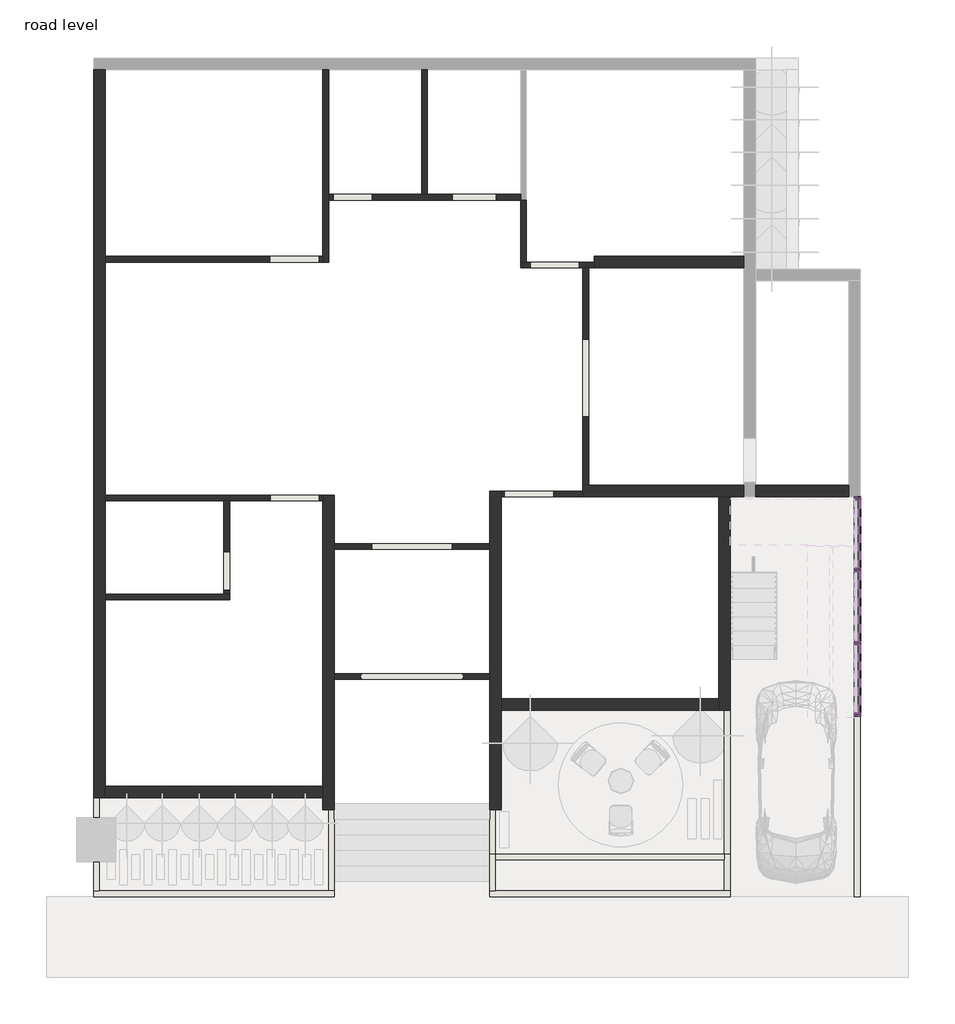
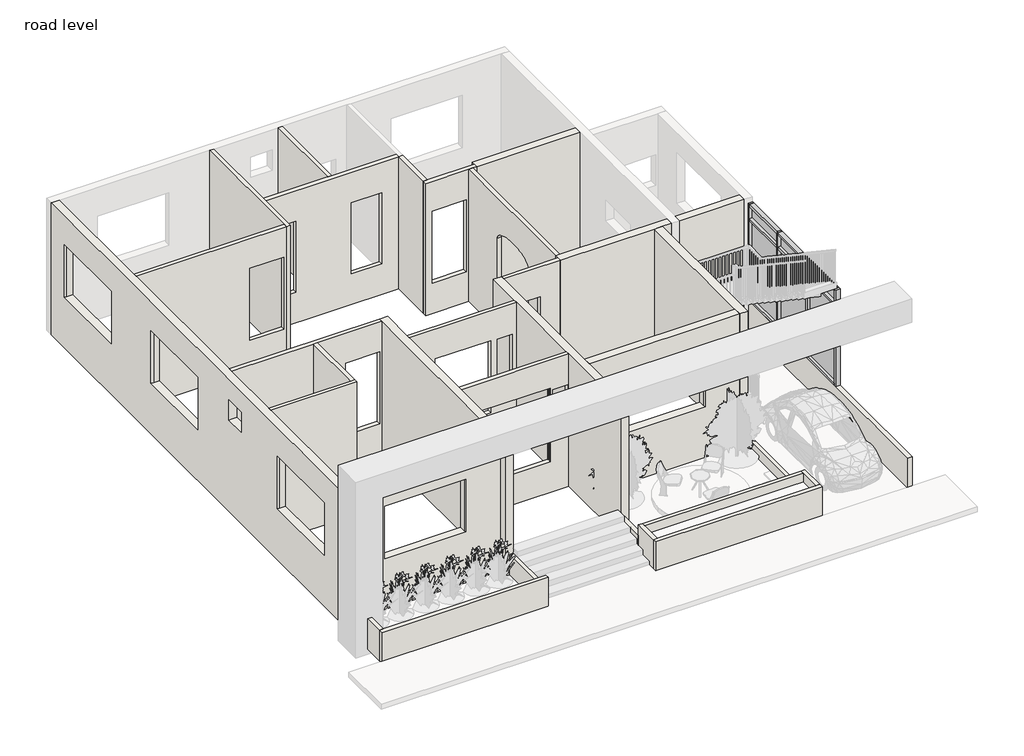
# One storey, part 1 of 3: 32 walls, 17 members, 6 plates.
"""IFC4 building model written with IfcOpenShell, lengths in millimetres."""

from ifc_helpers import new_model, si_unit, point, frame, origin, origin_with_axes, place, context, project, spatial, polyline, ellipse_curve, trimmed, outline, extrude, faceted_brep, transform, mapped, element, save
from ifc_brep_helpers import plane_surface, extruded_surface, advanced_brep
from components import member_97a07400, member_91c435ce, member_f0fea5a5, member_ffd4c858, member_64ac20db, member_08a74848, member_ee409385, member_15823cb3, system_panel_glazed_bd4b6abd, system_panel_glazed_9f7cb957, system_panel_glazed_bee7dd50, system_panel_glazed_ee0060d4

model = new_model("IFC4")

# Units and contexts
model_context = context("Model", 3, world=origin())
ifc_project = project(units=[si_unit("LENGTHUNIT", "METRE", prefix="MILLI")], contexts=[model_context])

# Site, building, storey
site = spatial("IfcSite", under=ifc_project)
building = spatial("IfcBuilding", under=site)
storey = spatial("IfcBuildingStorey", under=building, Name="road level", Elevation=0.0)

# Members
placement = place(None, origin())
member_shape = member_97a07400(model_context)
element("IfcMember", 1, ObjectType="Rectangular Mullion : 2.5\" x 5\" rectangular", at=placement, inside=storey, context=model_context, shape_type="MappedRepresentation", body=[
    mapped(member_shape, transform((-5177.1494093, 2444.9237487, 3810.0), x_axis=(0.0, 0.0, 1.0), y_axis=(-1.0, 0.0, 0.0), z_axis=(0.0, -1.0, 0.0))),
])
element("IfcMember", 2, ObjectType="Rectangular Mullion : 2.5\" x 5\" rectangular", at=placement, inside=storey, context=model_context, shape_type="MappedRepresentation", body=[
    mapped(member_shape, transform((-5177.1494093, 5283.3737486, 3810.0), x_axis=(0.0, 0.0, 1.0), y_axis=(-1.0, 0.0, 0.0), z_axis=(0.0, -1.0, 0.0))),
])
member_2_shape = member_91c435ce(model_context)
element("IfcMember", 3, ObjectType="Rectangular Mullion : 2.5\" x 5\" rectangular", at=placement, inside=storey, context=model_context, shape_type="MappedRepresentation", body=[
    mapped(member_2_shape, transform((-5177.1494093, 3848.2737488, 3810.0), x_axis=(0.0, 0.0, 1.0), y_axis=(-1.0, 0.0, 0.0), z_axis=(0.0, -1.0, 0.0))),
])
element("IfcMember", 4, ObjectType="Rectangular Mullion : 2.5\" x 5\" rectangular", at=placement, inside=storey, context=model_context, shape_type="MappedRepresentation", body=[
    mapped(member_shape, transform((-5177.1494093, 6623.2237487, 914.4), x_axis=(0.0, 0.0, -1.0), y_axis=(-1.0, 0.0, 0.0), z_axis=(0.0, 1.0, 0.0))),
])
element("IfcMember", 5, ObjectType="Rectangular Mullion : 2.5\" x 5\" rectangular", at=placement, inside=storey, context=model_context, shape_type="MappedRepresentation", body=[
    mapped(member_shape, transform((-5177.1494093, 3784.7737488, 914.4), x_axis=(0.0, 0.0, -1.0), y_axis=(-1.0, 0.0, 0.0), z_axis=(0.0, 1.0, 0.0))),
])
element("IfcMember", 6, ObjectType="Rectangular Mullion : 2.5\" x 5\" rectangular", at=placement, inside=storey, context=model_context, shape_type="MappedRepresentation", body=[
    mapped(member_2_shape, transform((-5177.1494093, 5219.8737486, 914.4), x_axis=(0.0, 0.0, -1.0), y_axis=(-1.0, 0.0, 0.0), z_axis=(0.0, 1.0, 0.0))),
])
member_3_shape = member_f0fea5a5(model_context)
element("IfcMember", 7, ObjectType="Rectangular Mullion : 2.5\" x 5\" rectangular", at=placement, inside=storey, context=model_context, shape_type="MappedRepresentation", body=[
    mapped(member_3_shape, transform((-5177.1494093, 5251.6237486, 914.4), x_axis=(0.0, -1.0, 0.0), y_axis=(-1.0, 0.0, 0.0), z_axis=(0.0, 0.0, -1.0))),
])
element("IfcMember", 8, ObjectType="Rectangular Mullion : 2.5\" x 5\" rectangular", at=placement, inside=storey, context=model_context, shape_type="MappedRepresentation", body=[
    mapped(member_3_shape, transform((-5177.1494093, 3816.5237488, 914.4), x_axis=(0.0, -1.0, 0.0), y_axis=(-1.0, 0.0, 0.0), z_axis=(0.0, 0.0, -1.0))),
])
member_4_shape = member_ffd4c858(model_context)
element("IfcMember", 9, ObjectType="Rectangular Mullion : 2.5\" x 5\" rectangular", at=placement, inside=storey, context=model_context, shape_type="MappedRepresentation", body=[
    mapped(member_4_shape, transform((-5177.1494093, 5251.6237486, 3352.8), x_axis=(0.0, -1.0, 0.0), y_axis=(-1.0, 0.0, 0.0), z_axis=(0.0, 0.0, -1.0))),
])
element("IfcMember", 10, ObjectType="Rectangular Mullion : 2.5\" x 5\" rectangular", at=placement, inside=storey, context=model_context, shape_type="MappedRepresentation", body=[
    mapped(member_4_shape, transform((-5177.1494093, 3816.5237488, 3352.8), x_axis=(0.0, -1.0, 0.0), y_axis=(-1.0, 0.0, 0.0), z_axis=(0.0, 0.0, -1.0))),
])
member_5_shape = member_64ac20db(model_context)
element("IfcMember", 11, ObjectType="Rectangular Mullion : 2.5\" x 5\" rectangular", at=placement, inside=storey, context=model_context, shape_type="MappedRepresentation", body=[
    mapped(member_5_shape, transform((-5177.1494093, 5283.3737486, 3352.8), x_axis=(0.0, 0.0, 1.0), y_axis=(-1.0, 0.0, 0.0), z_axis=(0.0, -1.0, 0.0))),
])
element("IfcMember", 12, ObjectType="Rectangular Mullion : 2.5\" x 5\" rectangular", at=placement, inside=storey, context=model_context, shape_type="MappedRepresentation", body=[
    mapped(member_5_shape, transform((-5177.1494093, 2444.9237487, 3352.8), x_axis=(0.0, 0.0, 1.0), y_axis=(-1.0, 0.0, 0.0), z_axis=(0.0, -1.0, 0.0))),
])
member_6_shape = member_08a74848(model_context)
element("IfcMember", 13, ObjectType="Rectangular Mullion : 2.5\" x 5\" rectangular", at=placement, inside=storey, context=model_context, shape_type="MappedRepresentation", body=[
    mapped(member_6_shape, transform((-5177.1494093, 3848.2737488, 3352.8), x_axis=(0.0, 0.0, 1.0), y_axis=(-1.0, 0.0, 0.0), z_axis=(0.0, -1.0, 0.0))),
])
member_7_shape = member_ee409385(model_context)
element("IfcMember", 14, ObjectType="Rectangular Mullion : 2.5\" x 5\" rectangular", at=placement, inside=storey, context=model_context, shape_type="MappedRepresentation", body=[
    mapped(member_7_shape, transform((-5177.1494093, 2381.4237487, 914.4), x_axis=(0.0, -1.0, 0.0), y_axis=(-1.0, 0.0, 0.0), z_axis=(0.0, 0.0, -1.0))),
])
member_8_shape = member_15823cb3(model_context)
element("IfcMember", 15, ObjectType="Rectangular Mullion : 2.5\" x 5\" rectangular", at=placement, inside=storey, context=model_context, shape_type="MappedRepresentation", body=[
    mapped(member_8_shape, transform((-5177.1494093, 6686.7237487, 3810.0), x_axis=(0.0, 1.0, 0.0), y_axis=(-1.0, 0.0, 0.0), z_axis=(0.0, 0.0, 1.0))),
])
element("IfcMember", 16, ObjectType="Rectangular Mullion : 2.5\" x 5\" rectangular", at=placement, inside=storey, context=model_context, shape_type="MappedRepresentation", body=[
    mapped(member_8_shape, transform((-5177.1494093, 2381.4237487, 3352.8), x_axis=(0.0, -1.0, 0.0), y_axis=(-1.0, 0.0, 0.0), z_axis=(0.0, 0.0, -1.0))),
])
element("IfcMember", 17, ObjectType="Rectangular Mullion : 2.5\" x 5\" rectangular", at=placement, inside=storey, context=model_context, shape_type="MappedRepresentation", body=[
    mapped(member_7_shape, transform((-5177.1494093, 6686.7237487, 3352.8), x_axis=(0.0, 1.0, 0.0), y_axis=(-1.0, 0.0, 0.0), z_axis=(0.0, 0.0, 1.0))),
])

# Plates
system_panel_glazed_shape = system_panel_glazed_bd4b6abd(model_context)
element("IfcPlate", 18, ObjectType="System Panel : Glazed", at=placement, inside=storey, context=model_context, shape_type="MappedRepresentation", body=[
    mapped(system_panel_glazed_shape, transform((-5177.1494093, 5953.2987486, 977.9), x_axis=(0.0, -1.0, 0.0), y_axis=(1.0, 0.0, 0.0), z_axis=(0.0, 0.0, 1.0))),
])
element("IfcPlate", 19, ObjectType="System Panel : Glazed", at=placement, inside=storey, context=model_context, shape_type="MappedRepresentation", body=[
    mapped(system_panel_glazed_shape, transform((-5177.1494093, 3114.8487487, 977.9), x_axis=(0.0, -1.0, 0.0), y_axis=(1.0, 0.0, 0.0), z_axis=(0.0, 0.0, 1.0))),
])
system_panel_glazed_2_shape = system_panel_glazed_9f7cb957(model_context)
element("IfcPlate", 20, ObjectType="System Panel : Glazed", at=placement, inside=storey, context=model_context, shape_type="MappedRepresentation", body=[
    mapped(system_panel_glazed_2_shape, transform((-5177.1494093, 4534.0737487, 977.9), x_axis=(0.0, -1.0, 0.0), y_axis=(1.0, 0.0, 0.0), z_axis=(0.0, 0.0, 1.0))),
])
system_panel_glazed_3_shape = system_panel_glazed_bee7dd50(model_context)
element("IfcPlate", 21, ObjectType="System Panel : Glazed", at=placement, inside=storey, context=model_context, shape_type="MappedRepresentation", body=[
    mapped(system_panel_glazed_3_shape, transform((-5177.1494093, 5953.2987486, 3384.55), x_axis=(0.0, -1.0, 0.0), y_axis=(1.0, 0.0, 0.0), z_axis=(0.0, 0.0, 1.0))),
])
element("IfcPlate", 22, ObjectType="System Panel : Glazed", at=placement, inside=storey, context=model_context, shape_type="MappedRepresentation", body=[
    mapped(system_panel_glazed_3_shape, transform((-5177.1494093, 3114.8487487, 3384.55), x_axis=(0.0, -1.0, 0.0), y_axis=(1.0, 0.0, 0.0), z_axis=(0.0, 0.0, 1.0))),
])
system_panel_glazed_4_shape = system_panel_glazed_ee0060d4(model_context)
element("IfcPlate", 23, ObjectType="System Panel : Glazed", at=placement, inside=storey, context=model_context, shape_type="MappedRepresentation", body=[
    mapped(system_panel_glazed_4_shape, transform((-5177.1494093, 4534.0737487, 3384.55), x_axis=(0.0, -1.0, 0.0), y_axis=(1.0, 0.0, 0.0), z_axis=(0.0, 0.0, 1.0))),
])

# Walls
element("IfcWall", 24, ObjectType="Generic - 4.5\"", at=placement, inside=storey, context=model_context, shape_type="Brep", body=[
    faceted_brep([(-15673.6994093, 15068.7237487, 0.0), (-15673.6994093, 11411.1237487, 0.0), (-15673.6994093, 11296.8237487, 0.0), (-15673.6994093, 11296.8237487, 3962.4), (-15673.6994093, 11411.1237487, 3962.4), (-15673.6994093, 15068.7237487, 3962.4), (-15559.3994093, 15068.7237487, 0.0), (-15559.3994093, 15068.7237487, 3962.4), (-15559.3994093, 12630.3237487, 3962.4), (-15559.3994093, 12516.0237487, 3962.4), (-15559.3994093, 11296.8237487, 3962.4), (-15559.3994093, 11296.8237487, 0.0), (-15559.3994093, 12516.0237487, 0.0), (-15559.3994093, 12630.3237487, 0.0)], [[[0, 1, 2, 3, 4, 5]], [[6, 7, 8, 9, 10, 11, 12, 13]], [[2, 1, 0, 6, 13, 12, 11]], [[0, 5, 7, 6]], [[3, 2, 11, 10]], [[5, 4, 3, 10, 9, 8, 7]]]),
])
element("IfcWall", 25, ObjectType="Generic - 4.5\"", at=placement, inside=storey, context=model_context, shape_type="SweptSolid", body=[
    extrude(outline(polyline([(0.0, -19940.8994093), (0.0, -15673.6994093), (3962.4, -15673.6994093), (3962.4, -19940.8994093), (0.0, -19940.8994093)]), holes=[polyline([(3073.4, -15743.5494093), (914.4, -15743.5494093), (914.4, -16708.7494093), (3073.4, -16708.7494093), (3073.4, -15743.5494093)])]), frame((0.0, 11296.8237487, 0.0), z_axis=(0.0, 1.0, 0.0), x_axis=(0.0, 0.0, 1.0)), (0.0, 0.0, 1.0), 114.3),
])
element("IfcWall", 26, ObjectType="Generic - 4.5\"", at=placement, inside=storey, context=model_context, shape_type="SweptSolid", body=[
    extrude(outline(polyline([(-13730.5994093, 12630.3237487), (-13730.5994093, 15068.7237487), (-13616.2994093, 15068.7237487), (-13616.2994093, 12630.3237487), (-13730.5994093, 12630.3237487)])), origin_with_axes(), (0.0, 0.0, 1.0), 3962.4),
])
element("IfcWall", 27, ObjectType="Generic - 4.5\"", at=placement, inside=storey, context=model_context, shape_type="Brep", body=[
    faceted_brep([(-11787.4994093, 12630.3237487, 0.0), (-13616.2994093, 12630.3237487, 0.0), (-13730.5994093, 12630.3237487, 0.0), (-15559.3994093, 12630.3237487, 0.0), (-15559.3994093, 12630.3237487, 3962.4), (-13730.5994093, 12630.3237487, 3962.4), (-13616.2994093, 12630.3237487, 3962.4), (-11787.4994093, 12630.3237487, 3962.4), (-13133.6994093, 12630.3237487, 3048.0), (-13133.6994093, 12630.3237487, 914.4), (-12270.0994093, 12630.3237487, 914.4), (-12270.0994093, 12630.3237487, 3048.0), (-14702.1494093, 12630.3237487, 914.4), (-14702.1494093, 12630.3237487, 3048.0), (-15464.1494093, 12630.3237487, 3048.0), (-15464.1494093, 12630.3237487, 914.4), (-11787.4994093, 12516.0237487, 0.0), (-11787.4994093, 12516.0237487, 3962.4), (-15559.3994093, 12516.0237487, 3962.4), (-15559.3994093, 12516.0237487, 0.0), (-13133.6994093, 12516.0237487, 3048.0), (-12270.0994093, 12516.0237487, 3048.0), (-12270.0994093, 12516.0237487, 914.4), (-13133.6994093, 12516.0237487, 914.4), (-14702.1494093, 12516.0237487, 914.4), (-15464.1494093, 12516.0237487, 914.4), (-15464.1494093, 12516.0237487, 3048.0), (-14702.1494093, 12516.0237487, 3048.0)], [[[0, 1, 2, 3, 4, 5, 6, 7], [8, 9, 10, 11], [12, 13, 14, 15]], [[16, 17, 18, 19], [20, 21, 22, 23], [24, 25, 26, 27]], [[3, 2, 1, 0, 16, 19]], [[4, 3, 19, 18]], [[0, 7, 17, 16]], [[9, 8, 20, 23]], [[10, 9, 23, 22]], [[11, 10, 22, 21]], [[8, 11, 21, 20]], [[25, 24, 12, 15]], [[26, 25, 15, 14]], [[27, 26, 14, 13]], [[24, 27, 13, 12]], [[7, 6, 5, 4, 18, 17]]]),
])
element("IfcWall", 28, ObjectType="Generic - 4.5\"", at=placement, inside=storey, context=model_context, shape_type="SweptSolid", body=[
    extrude(outline(polyline([(-11673.1994093, 12516.0237487), (-11673.1994093, 11296.8237487), (-11787.4994093, 11296.8237487), (-11787.4994093, 12516.0237487), (-11673.1994093, 12516.0237487)])), origin_with_axes(), (0.0, 0.0, 1.0), 3962.4),
])
element("IfcWall", 29, ObjectType="Generic - 4.5\"", at=placement, inside=storey, context=model_context, shape_type="Brep", body=[
    faceted_brep([(-19940.8994093, 6610.5237487, 0.0), (-17616.7994093, 6610.5237487, 0.0), (-17502.4994093, 6610.5237487, 0.0), (-15673.6994093, 6610.5237487, 0.0), (-15673.6994093, 6610.5237487, 3962.4), (-17502.4994093, 6610.5237487, 3962.4), (-17616.7994093, 6610.5237487, 3962.4), (-19940.8994093, 6610.5237487, 3962.4), (-15737.1994093, 6610.5237487, 3073.4), (-15737.1994093, 6610.5237487, 914.4), (-16702.3994093, 6610.5237487, 914.4), (-16702.3994093, 6610.5237487, 3073.4), (-15673.6994093, 6724.8237487, 0.0), (-19940.8994093, 6724.8237487, 0.0), (-19940.8994093, 6724.8237487, 3962.4), (-15673.6994093, 6724.8237487, 3962.4), (-15737.1994093, 6724.8237487, 914.4), (-15737.1994093, 6724.8237487, 3073.4), (-16702.3994093, 6724.8237487, 3073.4), (-16702.3994093, 6724.8237487, 914.4)], [[[0, 1, 2, 3, 4, 5, 6, 7], [8, 9, 10, 11]], [[12, 13, 14, 15], [16, 17, 18, 19]], [[3, 2, 1, 0, 13, 12]], [[0, 7, 14, 13]], [[4, 3, 12, 15]], [[16, 9, 8, 17]], [[17, 8, 11, 18]], [[18, 11, 10, 19]], [[9, 16, 19, 10]], [[7, 6, 5, 4, 15, 14]]]),
])
element("IfcWall", 30, ObjectType="Generic - 4.5\"", at=placement, inside=storey, context=model_context, shape_type="Brep", body=[
    faceted_brep([(-19940.8994093, 4667.4237487, 0.0), (-17502.4994093, 4667.4237487, 0.0), (-17502.4994093, 4667.4237487, 3962.4), (-19940.8994093, 4667.4237487, 3962.4), (-19940.8994093, 4781.7237487, 0.0), (-19940.8994093, 4781.7237487, 3962.4), (-17616.7994093, 4781.7237487, 3962.4), (-17502.4994093, 4781.7237487, 3962.4), (-17502.4994093, 4781.7237487, 0.0), (-17616.7994093, 4781.7237487, 0.0)], [[[0, 1, 2, 3]], [[4, 5, 6, 7, 8, 9]], [[1, 0, 4, 9, 8]], [[0, 3, 5, 4]], [[2, 1, 8, 7]], [[3, 2, 7, 6, 5]]]),
])
element("IfcWall", 31, ObjectType="Generic - 4.5\"", at=placement, inside=storey, context=model_context, shape_type="SweptSolid", body=[
    extrude(outline(polyline([(4781.7237487, 0.0), (4781.7237487, 3962.4), (6610.5237487, 3962.4), (6610.5237487, 0.0), (4781.7237487, 0.0)]), holes=[polyline([(5613.5737487, 914.4), (5613.5737487, 3048.0), (4851.5737487, 3048.0), (4851.5737487, 914.4), (5613.5737487, 914.4)])]), frame((-17616.7994093, 0.0, 0.0), z_axis=(1.0, 0.0, 0.0), x_axis=(0.0, 1.0, 0.0)), (0.0, 0.0, 1.0), 114.3),
])
element("IfcWall", 32, ObjectType="Generic - 4.5\"", at=placement, inside=storey, context=model_context, shape_type="Brep", body=[
    faceted_brep([(-10339.6994093, 11296.8237487, 0.0), (-11673.1994093, 11296.8237487, 0.0), (-11787.4994093, 11296.8237487, 0.0), (-11787.4994093, 11296.8237487, 3962.4), (-11673.1994093, 11296.8237487, 3962.4), (-10339.6994093, 11296.8237487, 3962.4), (-11603.3494093, 11296.8237487, 3073.4), (-11603.3494093, 11296.8237487, 914.4), (-10638.1494093, 11296.8237487, 914.4), (-10638.1494093, 11296.8237487, 3073.4), (-11787.4994093, 11182.5237487, 0.0), (-10568.2994093, 11182.5237487, 0.0), (-10453.9994093, 11182.5237487, 0.0), (-10339.6994093, 11182.5237487, 0.0), (-10339.6994093, 11182.5237487, 3962.4), (-10453.9994093, 11182.5237487, 3962.4), (-10568.2994093, 11182.5237487, 3962.4), (-11787.4994093, 11182.5237487, 3962.4), (-11603.3494093, 11182.5237487, 914.4), (-11603.3494093, 11182.5237487, 3073.4), (-10638.1494093, 11182.5237487, 3073.4), (-10638.1494093, 11182.5237487, 914.4)], [[[0, 1, 2, 3, 4, 5], [6, 7, 8, 9]], [[10, 11, 12, 13, 14, 15, 16, 17], [18, 19, 20, 21]], [[2, 1, 0, 13, 12, 11, 10]], [[0, 5, 14, 13]], [[3, 2, 10, 17]], [[18, 7, 6, 19]], [[19, 6, 9, 20]], [[20, 9, 8, 21]], [[7, 18, 21, 8]], [[5, 4, 3, 17, 16, 15, 14]]]),
])
element("IfcWall", 33, ObjectType="Generic - 4.5\"", at=placement, inside=storey, context=model_context, shape_type="AdvancedBrep", body=[
    advanced_brep(
    [(-10453.9994093, 6915.3237487, 0.0), (-10453.9994093, 11182.5237487, 0.0), (-10453.9994093, 11182.5237487, 3962.4), (-10453.9994093, 6915.3237487, 3962.4), (-10453.9994093, 8258.3487487, 2743.2), (-10453.9994093, 9782.3487487, 2743.2), (-10453.9994093, 9782.3487487, 914.4), (-10453.9994093, 8258.3487487, 914.4), (-10568.2994093, 6915.3237487, 0.0), (-10568.2994093, 6915.3237487, 3962.4), (-10568.2994093, 11182.5237487, 3962.4), (-10568.2994093, 11182.5237487, 0.0), (-10568.2994093, 8258.3487487, 2743.2), (-10568.2994093, 8258.3487487, 914.4), (-10568.2994093, 9782.3487487, 914.4), (-10568.2994093, 9782.3487487, 2743.2)],
    [
        (0, 1),
        (1, 2),
        (2, 3),
        (3, 0),
        (4, 5, ellipse_curve(frame((-10453.9994093, 9020.3487487, 2743.2), z_axis=(-1.0, 0.0, 0.0), x_axis=(0.0, -1.0, 0.0)), 762.0, 304.8)),
        (5, 6),
        (6, 7),
        (7, 4),
        (8, 9),
        (9, 10),
        (10, 11),
        (11, 8),
        (12, 13),
        (13, 14),
        (14, 15),
        (15, 12, ellipse_curve(frame((-10568.2994093, 9020.3487487, 2743.2), z_axis=(1.0, 0.0, 0.0), x_axis=(0.0, -1.0, 0.0)), 762.0, 304.8)),
        (0, 8),
        (11, 1),
        (3, 9),
        (10, 2),
        (4, 12),
        (15, 5),
        (14, 6),
        (13, 7),
    ],
    [
        plane_surface(frame((-10453.9994093, 7900.8437487, 0.0), z_axis=(1.0, 0.0, 0.0), x_axis=(0.0, 1.0, 0.0))),
        plane_surface(frame((-10568.2994093, 7900.8437487, 0.0), z_axis=(-1.0, 0.0, 0.0), x_axis=(0.0, -1.0, 0.0))),
        plane_surface(frame((-10453.9994093, 6743.8737487, 0.0), z_axis=(0.0, 0.0, -1.0), x_axis=(-1.0, 0.0, 0.0))),
        plane_surface(frame((-6738.5424924, 6915.3237487, 0.0), z_axis=(0.0, -1.0, 0.0), x_axis=(-1.0, 0.0, 0.0))),
        plane_surface(frame((-7691.7494093, 11182.5237487, 0.0), z_axis=(0.0, 1.0, 0.0), x_axis=(1.0, 0.0, 0.0))),
        extruded_surface(trimmed(ellipse_curve(frame((-10682.5994093, 9020.3487487, 2743.2), z_axis=(-1.0, 0.0, 0.0), x_axis=(0.0, -1.0, 0.0)), 762.0, 304.8), [point((-10682.5994093, 8258.3487487, 2743.2))], [point((-10682.5994093, 9782.3487487, 2743.2))], True, "CARTESIAN"), (114.30000000000109, 0.0, 0.0), 114.30000000000109),
        plane_surface(frame((-10453.9994093, 9782.3487487, 2743.2), z_axis=(0.0, -1.0, 0.0), x_axis=(-1.0, 0.0, 0.0))),
        plane_surface(frame((-10453.9994093, 9782.3487487, 914.4), z_axis=(0.0, 0.0, 1.0), x_axis=(-1.0, 0.0, 0.0))),
        plane_surface(frame((-10453.9994093, 8258.3487487, 914.4), z_axis=(0.0, 1.0, 0.0), x_axis=(-1.0, 0.0, 0.0))),
        plane_surface(frame((-6682.0994093, 15297.3237487, 3962.4), z_axis=(0.0, 0.0, 1.0), x_axis=(0.0, -1.0, 0.0))),
    ],
    [
        (0, [[1, 2, 3, 4], [5, 6, 7, 8]]),
        (1, [[9, 10, 11, 12], [13, 14, 15, 16]]),
        (2, [[-1, 17, -12, 18]]),
        (3, [[-4, 19, -9, -17]]),
        (4, [[-2, -18, -11, 20]]),
        (5, [[-5, 21, -16, 22]]),
        (6, [[-6, -22, -15, 23]]),
        (7, [[-7, -23, -14, 24]]),
        (8, [[-8, -24, -13, -21]]),
        (9, [[-3, -20, -10, -19]]),
    ],
),
])
element("IfcWall", 34, ObjectType="Generic - 4.5\"", at=placement, inside=storey, context=model_context, shape_type="SweptSolid", body=[
    extrude(outline(polyline([(0.0, -12168.4994093), (0.0, -10568.2994093), (3962.4, -10568.2994093), (3962.4, -12168.4994093), (0.0, -12168.4994093)]), holes=[polyline([(914.4, -12104.9994093), (3073.4, -12104.9994093), (3073.4, -11139.7994093), (914.4, -11139.7994093), (914.4, -12104.9994093)])]), frame((0.0, 6686.7237487, 0.0), z_axis=(0.0, 1.0, 0.0), x_axis=(0.0, 0.0, 1.0)), (0.0, 0.0, 1.0), 114.3),
])
element("IfcWall", 35, ObjectType="Generic - 4.5\"", at=placement, inside=storey, context=model_context, shape_type="SweptSolid", body=[
    extrude(outline(polyline([(-5234.2994093, -1161.8762513), (-5234.2994093, 6686.7237487), (-5119.9994093, 6686.7237487), (-5119.9994093, -1161.8762513), (-5234.2994093, -1161.8762513)])), origin_with_axes(), (0.0, 0.0, 1.0), 914.4),
])
element("IfcWall", 36, ObjectType="Generic - 4.5\"", at=placement, inside=storey, context=model_context, shape_type="Brep", body=[
    faceted_brep([(-7786.9994093, 2495.7237487, 0.0), (-7786.9994093, -323.6762513, 0.0), (-7786.9994093, -380.8262513, 0.0), (-7786.9994093, -380.8262513, 304.8), (-7786.9994093, -323.6762513, 304.8), (-7786.9994093, 2495.7237487, 304.8), (-7672.6994093, 2495.7237487, 0.0), (-7672.6994093, 2495.7237487, 304.8), (-7672.6994093, -323.6762513, 304.8), (-7672.6994093, -380.8262513, 304.8), (-7672.6994093, -380.8262513, 0.0)], [[[0, 1, 2, 3, 4, 5]], [[6, 7, 8, 9, 10]], [[2, 1, 0, 6, 10]], [[3, 2, 10, 9]], [[5, 4, 3, 9, 8, 7]], [[0, 5, 7, 6]]]),
])
element("IfcWall", 37, ObjectType="Generic - 4.5\"", at=placement, inside=storey, context=model_context, shape_type="SweptSolid", body=[
    extrude(outline(polyline([(-15559.3994093, -1047.5762513), (-15559.3994093, 546.2737487), (-15445.0994093, 546.2737487), (-15445.0994093, -1047.5762513), (-15559.3994093, -1047.5762513)])), origin_with_axes(), (0.0, 0.0, 1.0), 609.6),
])
element("IfcWall", 38, ObjectType="Generic - 4.5\"", at=placement, inside=storey, context=model_context, shape_type="SweptSolid", body=[
    extrude(outline(polyline([(-12397.0994093, -323.6762513), (-12397.0994093, 546.2737487), (-12282.7994093, 546.2737487), (-12282.7994093, -323.6762513), (-12397.0994093, -323.6762513)])), origin_with_axes(), (0.0, 0.0, 1.0), 609.6),
])
element("IfcWall", 39, ObjectType="Generic - 4.5\"", at=placement, inside=storey, context=model_context, shape_type="Brep", body=[
    faceted_brep([(-15445.0994093, -1047.5762513, 0.0), (-15559.3994093, -1047.5762513, 0.0), (-20055.1994093, -1047.5762513, 0.0), (-20169.4994093, -1047.5762513, 0.0), (-20169.4994093, -1047.5762513, 914.4), (-20055.1994093, -1047.5762513, 914.4), (-15445.0994093, -1047.5762513, 914.4), (-15445.0994093, -1047.5762513, 609.6), (-15445.0994093, -1161.8762513, 0.0), (-15445.0994093, -1161.8762513, 914.4), (-20169.4994093, -1161.8762513, 914.4), (-20169.4994093, -1161.8762513, 0.0)], [[[0, 1, 2, 3, 4, 5, 6, 7]], [[8, 9, 10, 11]], [[3, 2, 1, 0, 8, 11]], [[6, 5, 4, 10, 9]], [[4, 3, 11, 10]], [[0, 7, 6, 9, 8]]]),
])
element("IfcWall", 40, ObjectType="Generic - 4.5\"", at=placement, inside=storey, context=model_context, shape_type="SweptSolid", body=[
    extrude(outline(polyline([(-20169.4994093, -1047.5762513), (-20169.4994093, 781.2237487), (-20055.1994093, 781.2237487), (-20055.1994093, -1047.5762513), (-20169.4994093, -1047.5762513)])), origin_with_axes(), (0.0, 0.0, 1.0), 914.4),
])
element("IfcWall", 41, ObjectType="Generic - 4.5\"", at=placement, inside=storey, context=model_context, shape_type="Brep", body=[
    faceted_brep([(-12282.7994093, -437.9762513, 914.4), (-12282.7994093, -437.9762513, 0.0), (-7786.9994093, -437.9762513, 0.0), (-7786.9994093, -437.9762513, 914.4), (-12282.7994093, -323.6762513, 0.0), (-12282.7994093, -323.6762513, 914.4), (-7786.9994093, -323.6762513, 914.4), (-7786.9994093, -323.6762513, 304.8), (-7786.9994093, -323.6762513, 0.0), (-7786.9994093, -380.8262513, 0.0)], [[[0, 1, 2, 3]], [[4, 5, 6, 7, 8]], [[2, 1, 4, 8, 9]], [[0, 3, 6, 5]], [[2, 9, 8, 7, 6, 3]], [[0, 5, 4, 1]]]),
])
element("IfcWall", 42, ObjectType="Generic - 4.5\"", at=placement, inside=storey, context=model_context, shape_type="Brep", body=[
    faceted_brep([(-15445.0994093, 3105.3237487, 0.0), (-12397.0994093, 3105.3237487, 0.0), (-12397.0994093, 3105.3237487, 3962.4), (-15445.0994093, 3105.3237487, 3962.4), (-14921.0994093, 3105.3237487, 3123.4), (-12921.0994093, 3105.3237487, 3123.4), (-12921.0994093, 3105.3237487, 914.4), (-14921.0994093, 3105.3237487, 914.4), (-12854.2994093, 3105.3237487, 1828.8), (-12854.2994093, 3105.3237487, 3048.0), (-12422.4994093, 3105.3237487, 3048.0), (-12422.4994093, 3105.3237487, 1828.8), (-14987.8994093, 3105.3237487, 3048.0), (-14987.8994093, 3105.3237487, 1828.8), (-15419.6994093, 3105.3237487, 1828.8), (-15419.6994093, 3105.3237487, 3048.0), (-12397.0994093, 3219.6237487, 0.0), (-15445.0994093, 3219.6237487, 0.0), (-15445.0994093, 3219.6237487, 3962.4), (-12397.0994093, 3219.6237487, 3962.4), (-12921.0994093, 3219.6237487, 3123.4), (-14921.0994093, 3219.6237487, 3123.4), (-14921.0994093, 3219.6237487, 914.4), (-12921.0994093, 3219.6237487, 914.4), (-12854.2994093, 3219.6237487, 3048.0), (-12854.2994093, 3219.6237487, 1828.8), (-12422.4994093, 3219.6237487, 1828.8), (-12422.4994093, 3219.6237487, 3048.0), (-14987.8994093, 3219.6237487, 1828.8), (-14987.8994093, 3219.6237487, 3048.0), (-15419.6994093, 3219.6237487, 3048.0), (-15419.6994093, 3219.6237487, 1828.8), (-12921.0994093, 3199.6237487, 3123.4), (-14921.0994093, 3199.6237487, 3123.4), (-14921.0994093, 3129.6237487, 3123.4), (-12921.0994093, 3129.6237487, 3123.4), (-12921.0994093, 3129.6237487, 914.4), (-12906.0994093, 3129.6237487, 914.4), (-12906.0994093, 3199.6237487, 914.4), (-12921.0994093, 3199.6237487, 914.4), (-14921.0994093, 3199.6237487, 914.4), (-14936.0994093, 3199.6237487, 914.4), (-14936.0994093, 3129.6237487, 914.4), (-14921.0994093, 3129.6237487, 914.4), (-14936.0994093, 3129.6237487, 3138.4), (-12906.0994093, 3129.6237487, 3138.4), (-12906.0994093, 3199.6237487, 3138.4), (-14936.0994093, 3199.6237487, 3138.4)], [[[0, 1, 2, 3], [4, 5, 6, 7], [8, 9, 10, 11], [12, 13, 14, 15]], [[16, 17, 18, 19], [20, 21, 22, 23], [24, 25, 26, 27], [28, 29, 30, 31]], [[1, 0, 17, 16]], [[0, 3, 18, 17]], [[2, 1, 16, 19]], [[32, 33, 21, 20]], [[34, 35, 5, 4]], [[36, 37, 38, 39, 23, 22, 40, 41, 42, 43, 7, 6]], [[43, 34, 4, 7]], [[35, 36, 6, 5]], [[35, 34, 43, 42, 44, 45, 37, 36]], [[38, 37, 45, 46]], [[33, 32, 39, 38, 46, 47, 41, 40]], [[39, 32, 20, 23]], [[33, 40, 22, 21]], [[42, 41, 47, 44]], [[45, 44, 47, 46]], [[25, 24, 9, 8]], [[26, 25, 8, 11]], [[27, 26, 11, 10]], [[24, 27, 10, 9]], [[13, 12, 29, 28]], [[14, 13, 28, 31]], [[15, 14, 31, 30]], [[12, 15, 30, 29]], [[3, 2, 19, 18]]]),
])
element("IfcWall", 43, ObjectType="Generic - 4.5\"", at=placement, inside=storey, context=model_context, shape_type="SweptSolid", body=[
    extrude(outline(polyline([(0.0, -15445.0994093), (0.0, -12397.0994093), (3962.4, -12397.0994093), (3962.4, -15445.0994093), (0.0, -15445.0994093)]), holes=[polyline([(3073.4, -13133.6994093), (914.4, -13133.6994093), (914.4, -14708.4994093), (3073.4, -14708.4994093), (3073.4, -13133.6994093)]), polyline([(3048.0, -14860.8994093), (1828.8, -14860.8994093), (1828.8, -15292.6994093), (3048.0, -15292.6994093), (3048.0, -14860.8994093)]), polyline([(1828.8, -12955.8994093), (3048.0, -12955.8994093), (3048.0, -12524.0994093), (1828.8, -12524.0994093), (1828.8, -12955.8994093)])]), frame((0.0, 5658.0237487, 0.0), z_axis=(0.0, 1.0, 0.0), x_axis=(0.0, 0.0, 1.0)), (0.0, 0.0, 1.0), 114.3),
])
element("IfcWall", 44, ObjectType="Generic - 4.5\"", at=placement, inside=storey, context=model_context, shape_type="Brep", body=[
    faceted_brep([(-7672.6994093, -1047.5762513, 0.0), (-7786.9994093, -1047.5762513, 0.0), (-12282.7994093, -1047.5762513, 0.0), (-12397.0994093, -1047.5762513, 0.0), (-12397.0994093, -1047.5762513, 914.4), (-12282.7994093, -1047.5762513, 914.4), (-7786.9994093, -1047.5762513, 914.4), (-7672.6994093, -1047.5762513, 914.4), (-7672.6994093, -1161.8762513, 0.0), (-7672.6994093, -1161.8762513, 914.4), (-12397.0994093, -1161.8762513, 914.4), (-12397.0994093, -1161.8762513, 0.0)], [[[0, 1, 2, 3, 4, 5, 6, 7]], [[8, 9, 10, 11]], [[3, 2, 1, 0, 8, 11]], [[7, 6, 5, 4, 10, 9]], [[4, 3, 11, 10]], [[0, 7, 9, 8]]]),
])
element("IfcWall", 45, ObjectType="Generic - 4.5\"", at=placement, inside=storey, context=model_context, shape_type="Brep", body=[
    faceted_brep([(-7786.9994093, -380.8262513, 0.0), (-7786.9994093, -437.9762513, 0.0), (-7786.9994093, -1047.5762513, 0.0), (-7786.9994093, -1047.5762513, 914.4), (-7786.9994093, -437.9762513, 914.4), (-7786.9994093, -323.6762513, 914.4), (-7786.9994093, -323.6762513, 304.8), (-7786.9994093, -380.8262513, 304.8), (-7672.6994093, -380.8262513, 0.0), (-7672.6994093, -380.8262513, 304.8), (-7672.6994093, -323.6762513, 304.8), (-7672.6994093, -323.6762513, 914.4), (-7672.6994093, -1047.5762513, 914.4), (-7672.6994093, -1047.5762513, 0.0)], [[[0, 1, 2, 3, 4, 5, 6, 7]], [[8, 9, 10, 11, 12, 13]], [[2, 1, 0, 8, 13]], [[5, 4, 3, 12, 11]], [[3, 2, 13, 12]], [[0, 7, 9, 8]], [[6, 10, 9, 7]], [[6, 5, 11, 10]]]),
])
element("IfcWall", 46, ObjectType="Generic - 4.5\"", at=placement, inside=storey, context=model_context, shape_type="Brep", body=[
    faceted_brep([(-12397.0994093, -323.6762513, 0.0), (-12397.0994093, -1047.5762513, 0.0), (-12397.0994093, -1047.5762513, 914.4), (-12397.0994093, -323.6762513, 914.4), (-12397.0994093, -323.6762513, 609.6), (-12282.7994093, -323.6762513, 0.0), (-12282.7994093, -323.6762513, 609.6), (-12282.7994093, -323.6762513, 914.4), (-12282.7994093, -437.9762513, 914.4), (-12282.7994093, -1047.5762513, 914.4), (-12282.7994093, -1047.5762513, 0.0), (-12282.7994093, -437.9762513, 0.0)], [[[0, 1, 2, 3, 4]], [[5, 6, 7, 8, 9, 10, 11]], [[1, 0, 5, 11, 10]], [[3, 2, 9, 8, 7]], [[0, 4, 3, 7, 6, 5]], [[2, 1, 10, 9]]]),
])
element("IfcWall", 47, ObjectType="Generic - 9\"", at=placement, inside=storey, context=model_context, shape_type="Brep", body=[
    faceted_brep([(-20169.4994093, 15068.7237487, 0.0), (-20169.4994093, 781.2237487, 0.0), (-20169.4994093, 781.2237487, 914.4), (-20169.4994093, 781.2237487, 3962.4), (-20169.4994093, 15068.7237487, 3962.4), (-20169.4994093, 14423.6280739, 3098.8), (-20169.4994093, 12113.3694235, 3098.8), (-20169.4994093, 12113.3694235, 1524.0), (-20169.4994093, 14423.6280739, 1524.0), (-20169.4994093, 10165.9530739, 3098.8), (-20169.4994093, 7855.6944235, 3098.8), (-20169.4994093, 7855.6944235, 1524.0), (-20169.4994093, 10165.9530739, 1524.0), (-20169.4994093, 3965.1780739, 3098.8), (-20169.4994093, 1654.9194235, 3098.8), (-20169.4994093, 1654.9194235, 1524.0), (-20169.4994093, 3965.1780739, 1524.0), (-20169.4994093, 5727.8737487, 3352.8), (-20169.4994093, 5727.8737487, 2743.2), (-20169.4994093, 6337.4737487, 2743.2), (-20169.4994093, 6337.4737487, 3352.8), (-19940.8994093, 15068.7237487, 0.0), (-19940.8994093, 15068.7237487, 3962.4), (-19940.8994093, 11411.1237487, 3962.4), (-19940.8994093, 11296.8237487, 3962.4), (-19940.8994093, 6724.8237487, 3962.4), (-19940.8994093, 6610.5237487, 3962.4), (-19940.8994093, 4781.7237487, 3962.4), (-19940.8994093, 4667.4237487, 3962.4), (-19940.8994093, 1009.8237487, 3962.4), (-19940.8994093, 781.2237487, 3962.4), (-19940.8994093, 781.2237487, 0.0), (-19940.8994093, 1009.8237487, 0.0), (-19940.8994093, 4667.4237487, 0.0), (-19940.8994093, 4781.7237487, 0.0), (-19940.8994093, 6610.5237487, 0.0), (-19940.8994093, 6724.8237487, 0.0), (-19940.8994093, 11296.8237487, 0.0), (-19940.8994093, 11411.1237487, 0.0), (-19940.8994093, 12125.4987487, 3098.8), (-19940.8994093, 14411.4987487, 3098.8), (-19940.8994093, 14411.4987487, 1524.0), (-19940.8994093, 12125.4987487, 1524.0), (-19940.8994093, 7867.8237487, 3098.8), (-19940.8994093, 10153.8237487, 3098.8), (-19940.8994093, 10153.8237487, 1524.0), (-19940.8994093, 7867.8237487, 1524.0), (-19940.8994093, 1667.0487487, 3098.8), (-19940.8994093, 3953.0487487, 3098.8), (-19940.8994093, 3953.0487487, 1524.0), (-19940.8994093, 1667.0487487, 1524.0), (-19940.8994093, 5727.8737487, 3352.8), (-19940.8994093, 6337.4737487, 3352.8), (-19940.8994093, 6337.4737487, 2743.2), (-19940.8994093, 5727.8737487, 2743.2), (-20055.1994093, 781.2237487, 0.0), (-20100.7105877, 12125.4987487, 3098.8), (-20100.7105877, 14411.4987487, 3098.8), (-20100.7105877, 12125.4987487, 1524.0), (-20100.7105877, 14411.4987487, 1524.0), (-20100.7105877, 7867.8237487, 3098.8), (-20100.7105877, 10153.8237487, 3098.8), (-20100.7105877, 7867.8237487, 1524.0), (-20100.7105877, 10153.8237487, 1524.0), (-20100.7105877, 1667.0487487, 3098.8), (-20100.7105877, 3953.0487487, 3098.8), (-20100.7105877, 1667.0487487, 1524.0), (-20100.7105877, 3953.0487487, 1524.0)], [[[0, 1, 2, 3, 4], [5, 6, 7, 8], [9, 10, 11, 12], [13, 14, 15, 16], [17, 18, 19, 20]], [[21, 22, 23, 24, 25, 26, 27, 28, 29, 30, 31, 32, 33, 34, 35, 36, 37, 38], [39, 40, 41, 42], [43, 44, 45, 46], [47, 48, 49, 50], [51, 52, 53, 54]], [[1, 0, 21, 38, 37, 36, 35, 34, 33, 32, 31, 55]], [[0, 4, 22, 21]], [[1, 55, 31, 30, 3, 2]], [[56, 6, 5, 57, 40, 39]], [[58, 42, 41, 59, 8, 7]], [[56, 39, 42, 58]], [[40, 57, 59, 41]], [[57, 5, 8, 59]], [[6, 56, 58, 7]], [[60, 10, 9, 61, 44, 43]], [[62, 46, 45, 63, 12, 11]], [[60, 43, 46, 62]], [[44, 61, 63, 45]], [[61, 9, 12, 63]], [[10, 60, 62, 11]], [[64, 14, 13, 65, 48, 47]], [[66, 50, 49, 67, 16, 15]], [[64, 47, 50, 66]], [[48, 65, 67, 49]], [[65, 13, 16, 67]], [[14, 64, 66, 15]], [[18, 17, 51, 54]], [[19, 18, 54, 53]], [[20, 19, 53, 52]], [[17, 20, 52, 51]], [[4, 3, 30, 29, 28, 27, 26, 25, 24, 23, 22]]]),
])
element("IfcWall", 48, ObjectType="Generic - 9\"", at=placement, inside=storey, context=model_context, shape_type="Brep", body=[
    faceted_brep([(-19940.8994093, 781.2237487, 3962.4), (-19940.8994093, 781.2237487, 0.0), (-15673.6994093, 781.2237487, 0.0), (-15673.6994093, 781.2237487, 3962.4), (-18962.4287345, 781.2237487, 3098.8), (-16652.1700841, 781.2237487, 3098.8), (-16652.1700841, 781.2237487, 1524.0), (-18962.4287345, 781.2237487, 1524.0), (-19940.8994093, 1009.8237487, 0.0), (-19940.8994093, 1009.8237487, 3962.4), (-15673.6994093, 1009.8237487, 3962.4), (-15673.6994093, 1009.8237487, 0.0), (-16664.2994093, 1009.8237487, 3098.8), (-18950.2994093, 1009.8237487, 3098.8), (-18950.2994093, 1009.8237487, 1524.0), (-16664.2994093, 1009.8237487, 1524.0), (-16664.2994093, 850.0125702, 3098.8), (-18950.2994093, 850.0125702, 3098.8), (-16664.2994093, 850.0125702, 1524.0), (-18950.2994093, 850.0125702, 1524.0)], [[[0, 1, 2, 3], [4, 5, 6, 7]], [[8, 9, 10, 11], [12, 13, 14, 15]], [[2, 1, 8, 11]], [[3, 2, 11, 10]], [[0, 9, 8, 1]], [[16, 5, 4, 17, 13, 12]], [[18, 15, 14, 19, 7, 6]], [[16, 12, 15, 18]], [[13, 17, 19, 14]], [[17, 4, 7, 19]], [[5, 16, 18, 6]], [[0, 3, 10, 9]]]),
])
element("IfcWall", 49, ObjectType="Generic - 9\"", at=placement, inside=storey, context=model_context, shape_type="Brep", body=[
    faceted_brep([(-15445.0994093, 546.2737487, 0.0), (-15445.0994093, 3105.3237487, 0.0), (-15445.0994093, 3219.6237487, 0.0), (-15445.0994093, 5658.0237487, 0.0), (-15445.0994093, 5772.3237487, 0.0), (-15445.0994093, 6724.8237487, 0.0), (-15445.0994093, 6724.8237487, 3962.4), (-15445.0994093, 5772.3237487, 3962.4), (-15445.0994093, 5658.0237487, 3962.4), (-15445.0994093, 3219.6237487, 3962.4), (-15445.0994093, 3105.3237487, 3962.4), (-15445.0994093, 546.2737487, 3962.4), (-15445.0994093, 546.2737487, 609.6), (-15673.6994093, 546.2737487, 0.0), (-15673.6994093, 546.2737487, 3962.4), (-15673.6994093, 781.2237487, 3962.4), (-15673.6994093, 1009.8237487, 3962.4), (-15673.6994093, 6610.5237487, 3962.4), (-15673.6994093, 6724.8237487, 3962.4), (-15673.6994093, 6724.8237487, 0.0), (-15673.6994093, 6610.5237487, 0.0), (-15673.6994093, 1009.8237487, 0.0), (-15673.6994093, 781.2237487, 0.0), (-15559.3994093, 546.2737487, 0.0)], [[[0, 1, 2, 3, 4, 5, 6, 7, 8, 9, 10, 11, 12]], [[13, 14, 15, 16, 17, 18, 19, 20, 21, 22]], [[5, 4, 3, 2, 1, 0, 23, 13, 22, 21, 20, 19]], [[0, 12, 11, 14, 13, 23]], [[6, 5, 19, 18]], [[11, 10, 9, 8, 7, 6, 18, 17, 16, 15, 14]]]),
])
element("IfcWall", 50, ObjectType="Generic - 9\"", at=placement, inside=storey, context=model_context, shape_type="Brep", body=[
    faceted_brep([(-7405.9994093, 6915.3237487, 0.0), (-10453.9994093, 6915.3237487, 0.0), (-10568.2994093, 6915.3237487, 0.0), (-10568.2994093, 6915.3237487, 3962.4), (-10453.9994093, 6915.3237487, 3962.4), (-7405.9994093, 6915.3237487, 3962.4), (-7405.9994093, 6686.7237487, 0.0), (-7405.9994093, 6686.7237487, 3962.4), (-7672.6994093, 6686.7237487, 3962.4), (-7901.2994093, 6686.7237487, 3962.4), (-10568.2994093, 6686.7237487, 3962.4), (-10568.2994093, 6686.7237487, 0.0), (-7901.2994093, 6686.7237487, 0.0), (-7672.6994093, 6686.7237487, 0.0), (-10568.2994093, 6801.0237487, 0.0), (-10568.2994093, 6801.0237487, 3962.4)], [[[0, 1, 2, 3, 4, 5]], [[6, 7, 8, 9, 10, 11, 12, 13]], [[2, 1, 0, 6, 13, 12, 11, 14]], [[0, 5, 7, 6]], [[3, 2, 14, 11, 10, 15]], [[5, 4, 3, 15, 10, 9, 8, 7]]]),
])
element("IfcWall", 51, ObjectType="Generic - 9\"", at=placement, inside=storey, context=model_context, shape_type="Brep", body=[
    faceted_brep([(-7405.9994093, 11411.1237487, 0.0), (-10339.6994093, 11411.1237487, 0.0), (-10339.6994093, 11411.1237487, 3962.4), (-7405.9994093, 11411.1237487, 3962.4), (-7405.9994093, 11182.5237487, 0.0), (-7405.9994093, 11182.5237487, 3962.4), (-10339.6994093, 11182.5237487, 3962.4), (-10339.6994093, 11182.5237487, 0.0), (-10339.6994093, 11296.8237487, 0.0), (-10339.6994093, 11296.8237487, 3962.4)], [[[0, 1, 2, 3]], [[4, 5, 6, 7]], [[1, 0, 4, 7, 8]], [[2, 1, 8, 7, 6, 9]], [[0, 3, 5, 4]], [[3, 2, 9, 6, 5]]]),
])
element("IfcWall", 52, ObjectType="Generic - 9\"", at=placement, inside=storey, context=model_context, shape_type="Brep", body=[
    faceted_brep([(-12168.4994093, 546.2737487, 0.0), (-12168.4994093, 2495.7237487, 0.0), (-12168.4994093, 2724.3237487, 0.0), (-12168.4994093, 6686.7237487, 0.0), (-12168.4994093, 6801.0237487, 0.0), (-12168.4994093, 6801.0237487, 3962.4), (-12168.4994093, 6686.7237487, 3962.4), (-12168.4994093, 2724.3237487, 3962.4), (-12168.4994093, 2495.7237487, 3962.4), (-12168.4994093, 546.2737487, 3962.4), (-12397.0994093, 546.2737487, 0.0), (-12397.0994093, 546.2737487, 609.6), (-12397.0994093, 546.2737487, 3962.4), (-12397.0994093, 3105.3237487, 3962.4), (-12397.0994093, 3219.6237487, 3962.4), (-12397.0994093, 5658.0237487, 3962.4), (-12397.0994093, 5772.3237487, 3962.4), (-12397.0994093, 6801.0237487, 3962.4), (-12397.0994093, 6801.0237487, 0.0), (-12397.0994093, 5772.3237487, 0.0), (-12397.0994093, 5658.0237487, 0.0), (-12397.0994093, 3219.6237487, 0.0), (-12397.0994093, 3105.3237487, 0.0), (-12282.7994093, 546.2737487, 0.0)], [[[0, 1, 2, 3, 4, 5, 6, 7, 8, 9]], [[10, 11, 12, 13, 14, 15, 16, 17, 18, 19, 20, 21, 22]], [[4, 3, 2, 1, 0, 23, 10, 22, 21, 20, 19, 18]], [[0, 9, 12, 11, 10, 23]], [[5, 4, 18, 17]], [[9, 8, 7, 6, 5, 17, 16, 15, 14, 13, 12]]]),
])
element("IfcWall", 53, ObjectType="Generic - 9\"", at=placement, inside=storey, context=model_context, shape_type="Brep", body=[
    faceted_brep([(-7901.2994093, 6686.7237487, 0.0), (-7901.2994093, 2724.3237487, 0.0), (-7901.2994093, 2495.7237487, 0.0), (-7901.2994093, 2495.7237487, 3962.4), (-7901.2994093, 2724.3237487, 3962.4), (-7901.2994093, 6686.7237487, 3962.4), (-7672.6994093, 6686.7237487, 0.0), (-7672.6994093, 6686.7237487, 3962.4), (-7672.6994093, 6648.6237487, 3962.4), (-7672.6994093, 3499.0237487, 3962.4), (-7672.6994093, 2495.7237487, 3962.4), (-7672.6994093, 2495.7237487, 304.8), (-7672.6994093, 2495.7237487, 0.0), (-7786.9994093, 2495.7237487, 0.0)], [[[0, 1, 2, 3, 4, 5]], [[6, 7, 8, 9, 10, 11, 12]], [[2, 1, 0, 6, 12, 13]], [[0, 5, 7, 6]], [[2, 13, 12, 11, 10, 3]], [[5, 4, 3, 10, 9, 8, 7]]]),
])
element("IfcWall", 54, ObjectType="Generic - 9\"", at=placement, inside=storey, context=model_context, shape_type="Brep", body=[
    faceted_brep([(-7901.2994093, 2724.3237487, 3962.4), (-7901.2994093, 2724.3237487, 0.0), (-12168.4994093, 2724.3237487, 0.0), (-12168.4994093, 2724.3237487, 3962.4), (-8891.8994093, 2724.3237487, 3098.8), (-11177.8994093, 2724.3237487, 3098.8), (-11177.8994093, 2724.3237487, 1524.0), (-8891.8994093, 2724.3237487, 1524.0), (-7901.2994093, 2495.7237487, 0.0), (-7901.2994093, 2495.7237487, 3962.4), (-12168.4994093, 2495.7237487, 3962.4), (-12168.4994093, 2495.7237487, 0.0), (-11190.0287345, 2495.7237487, 3098.8), (-8879.7700841, 2495.7237487, 3098.8), (-8879.7700841, 2495.7237487, 1524.0), (-11190.0287345, 2495.7237487, 1524.0), (-8891.8994093, 2564.5125702, 3098.8), (-11177.8994093, 2564.5125702, 3098.8), (-8891.8994093, 2564.5125702, 1524.0), (-11177.8994093, 2564.5125702, 1524.0)], [[[0, 1, 2, 3], [4, 5, 6, 7]], [[8, 9, 10, 11], [12, 13, 14, 15]], [[2, 1, 8, 11]], [[3, 2, 11, 10]], [[0, 9, 8, 1]], [[16, 13, 12, 17, 5, 4]], [[18, 7, 6, 19, 15, 14]], [[16, 4, 7, 18]], [[5, 17, 19, 6]], [[17, 12, 15, 19]], [[13, 16, 18, 14]], [[0, 3, 10, 9]]]),
])
element("IfcWall", 55, ObjectType="Generic - 9\"", at=placement, inside=storey, context=model_context, shape_type="SweptSolid", body=[
    extrude(outline(polyline([(-5348.5994093, 6686.7237487), (-7177.3994093, 6686.7237487), (-7177.3994093, 6915.3237487), (-5348.5994093, 6915.3237487), (-5348.5994093, 6686.7237487)])), origin_with_axes(), (0.0, 0.0, 1.0), 3962.4),
])

save(model, "model.ifc")

# Revit data of these elements
# Type "Rectangular Mullion : 2.5\" x 5\" rectangular"
#   built-in parameter 1007304 = 0.416667 (stored number, unit not read)
#   built-in parameter 1007301 = 0.104167 (stored number, unit not read)
#   built-in parameter 1007300 = 0.104167 (stored number, unit not read)
# Type "System Panel : Glazed"
#   Construction Type Id = "GSP4R"
#   Analytic Construction = "1/8 in Pilkington single glazing"
#   Visual Light Transmittance = 0.9
#   Solar Heat Gain Coefficient = 0.86
#   Heat Transfer Coefficient (U) = 1.18115 BTU/(h·ft²·°F)
#   Define Thermal Properties by = 1
# Type "Generic - 4.5\""
#   Assembly Code = "B2010"
#   Layers, outside or top first: 0' - 4 1/2" no material (function 1)
# Type "Generic - 9\""
#   Assembly Code = "B2010"
#   Layers, outside or top first: 0' - 9" "Brick, Soldier Course" (function 1)
# Elements 1, 2, 3, 4, 5, 6, 7, 8, 9, 10, 11, 12, 13, 14, 15, 16, 17 (IfcMember, "Rectangular Mullion : 2.5\" x 5\" rectangular")
#   Phase Created = New Construction
#   Materials on its faces: "Aluminum"
# Elements 18, 19, 20, 21, 22, 23 (IfcPlate, "System Panel : Glazed")
#   Phase Created = New Construction
#   Materials on its faces: "Glass"
# Elements 24, 25, 26, 27, 28, 29, 30, 31, 32, 33, 34, 42, 43 (IfcWall, "Generic - 4.5\"")
#   Top Offset = 0' - 0"
#   Base Offset = 0' - 0"
#   wall height = 13' - 0"
#   Phase Created = New Construction
#   Base Constraint = road level
#   Top Constraint = 1st floor
#   Materials on its faces: "Default Wall"
# Elements 35, 39, 40, 45, 46 (IfcWall, "Generic - 4.5\"")
#   Top Offset = 0' - 0"
#   Base Offset = 0' - 0"
#   Unconnected Height = 3' - 0"
#   wall height = 3' - 0"
#   Phase Created = New Construction
#   Base Constraint = road level
#   Materials on its faces: "Default Wall"
# Element 36 (IfcWall, "Generic - 4.5\"")
#   Top Offset = 0' - 0"
#   Base Offset = 0' - 0"
#   Unconnected Height = 1' - 0"
#   wall height = 1' - 0"
#   Phase Created = New Construction
#   Base Constraint = road level
#   Materials on its faces: "Default Wall"
# Elements 37, 38 (IfcWall, "Generic - 4.5\"")
#   Top Offset = 0' - 0"
#   Base Offset = 0' - 0"
#   Unconnected Height = 2' - 0"
#   wall height = 2' - 0"
#   Phase Created = New Construction
#   Base Constraint = road level
#   Materials on its faces: "Default Wall"
# Elements 41, 44 (IfcWall, "Generic - 4.5\"")
#   Top Offset = 0' - 0"
#   Base Offset = 0' - 0"
#   wall height = 3' - 0"
#   Phase Created = New Construction
#   Base Constraint = road level
#   Materials on its faces: "Default Wall"
# Elements 47, 48, 51, 53, 54, 55 (IfcWall, "Generic - 9\"")
#   Top Offset = 0' - 0"
#   Base Offset = 0' - 0"
#   wall height = 13' - 0"
#   Phase Created = New Construction
#   Base Constraint = road level
#   Top Constraint = 1st floor
#   Materials on its faces: "Brick, Soldier Course"
# Elements 49, 50, 52 (IfcWall, "Generic - 9\"")
#   Top Offset = 0' - 0"
#   Base Offset = 0' - 0"
#   wall height = 13' - 0"
#   Phase Created = New Construction
#   Base Constraint = road level
#   Top Constraint = 1st floor
#   Materials on its faces: "Brick, Soldier Course", "Default Wall"
# Materials
#   "Brick, Soldier Course": class "Masonry", colour RGB 170 98 104, transparency 0, Description = "Common brick soldier coursed", Cost = 0
#   "Aluminum": class "Metal", colour RGB 247 247 247, transparency 0, Description = "Aluminum 6061", Cost = 0
#   "Glass": class "Glass", colour RGB 0 128 192, transparency 0.75, Description = "Soda Lime Glass", Cost = 0
#   "Default Wall": colour RGB 128 128 128, transparency 0, Cost = 0
